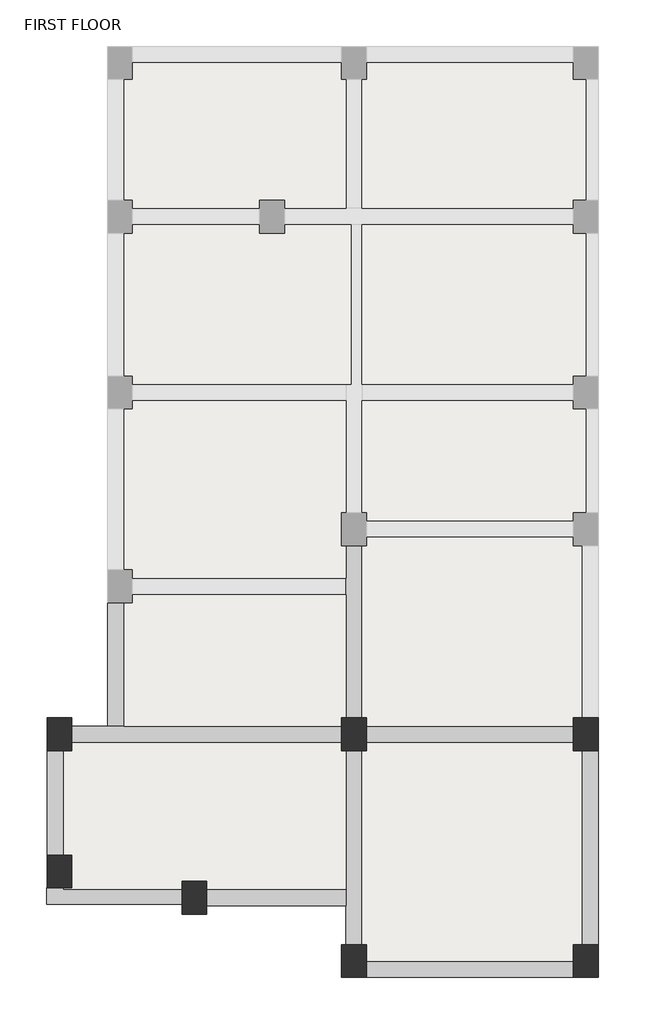
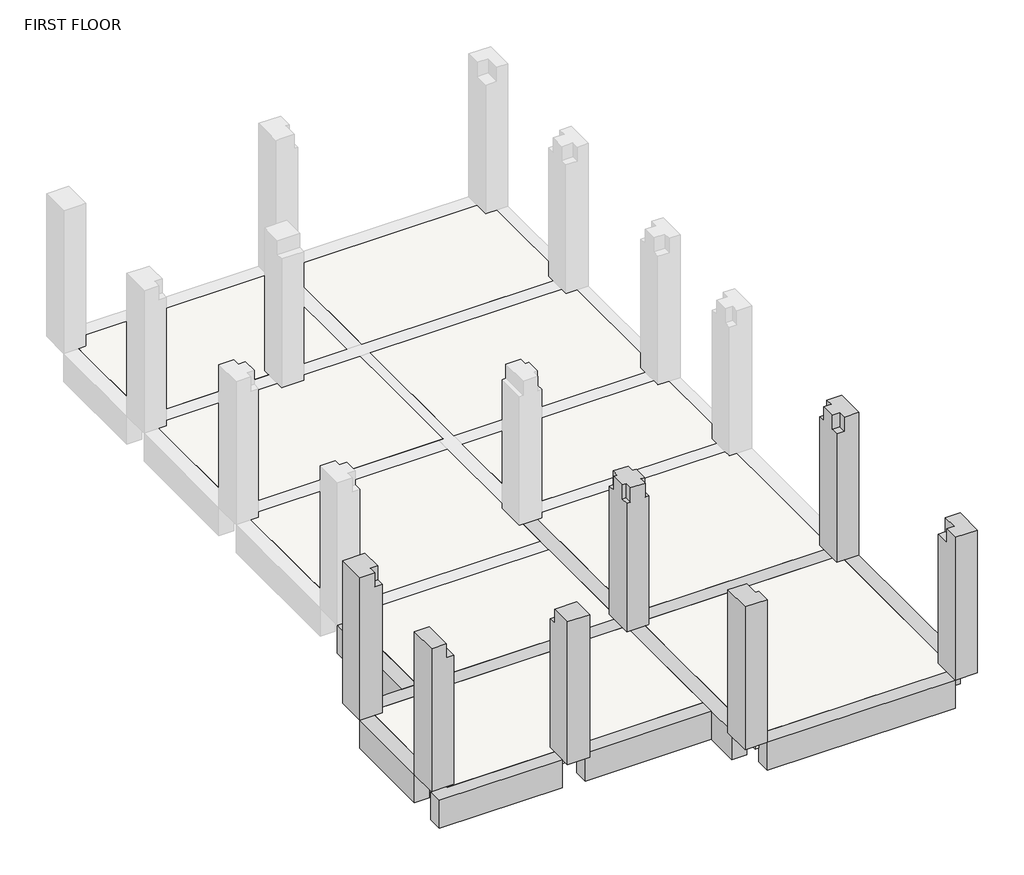
# One storey, part 1 of 2: 10 beams, 10 slabs, 7 columns.
"""IFC4 building model written with IfcOpenShell, lengths in millimetres."""

from ifc_helpers import new_model, si_unit, frame, origin, place, context, project, spatial, polyline, outline, extrude, faceted_brep, element, save

model = new_model("IFC4")

# Units and contexts
model_context = context("Model", 3, world=origin())
ifc_project = project(units=[si_unit("LENGTHUNIT", "METRE", prefix="MILLI")], contexts=[model_context])

# Site, building, storey
site = spatial("IfcSite", under=ifc_project)
building = spatial("IfcBuilding", under=site)
storey = spatial("IfcBuildingStorey", under=building, Name="FIRST FLOOR", Elevation=3000.0)

# Beams
placement = place(None, origin())
element("IfcBeam", 1, ObjectType="M_Concrete-Rectangular Beam : 300 x 600mm", at=placement, inside=storey, context=model_context, shape_type="SweptSolid", body=[
    extrude(outline(polyline([(2143.5134108, -6267.3380763), (2143.5134108, -6567.3380763), (-1646.635935, -6567.3380763), (-1646.635935, -6267.3380763), (2143.5134108, -6267.3380763)])), frame((0.0, 0.0, 2400.0), z_axis=(0.0, 0.0, 1.0), x_axis=(1.0, 0.0, 0.0)), (0.0, 0.0, 1.0), 600.0),
])
element("IfcBeam", 2, ObjectType="M_Concrete-Rectangular Beam : 300 x 600mm", at=placement, inside=storey, context=model_context, shape_type="SweptSolid", body=[
    extrude(outline(polyline([(2293.5134108, -2423.3693625), (2593.5134108, -2423.3693625), (2593.5134108, -5967.3380763), (2293.5134108, -5967.3380763), (2293.5134108, -2423.3693625)])), frame((0.0, 0.0, 2400.0), z_axis=(0.0, 0.0, 1.0), x_axis=(1.0, 0.0, 0.0)), (0.0, 0.0, 1.0), 600.0),
])
element("IfcBeam", 3, ObjectType="M_Concrete-Rectangular Beam : 300 x 600mm", at=placement, inside=storey, context=model_context, shape_type="SweptSolid", body=[
    extrude(outline(polyline([(-1646.635935, -2273.3693625), (-1646.635935, -1973.3693625), (2143.5134108, -1973.3693625), (2143.5134108, -2273.3693625), (-1646.635935, -2273.3693625)])), frame((0.0, 0.0, 2400.0), z_axis=(0.0, 0.0, 1.0), x_axis=(1.0, 0.0, 0.0)), (0.0, 0.0, 1.0), 600.0),
])
element("IfcBeam", 4, ObjectType="M_Concrete-Rectangular Beam : 300 x 600mm", at=placement, inside=storey, context=model_context, shape_type="Brep", body=[
    faceted_brep([(-1721.635935, -2423.3693625, 3000.0), (-2021.635935, -2423.3693625, 3000.0), (-2021.635935, -4959.2575036, 3000.0), (-2021.635935, -5259.2575036, 3000.0), (-2021.635935, -5967.3380763, 3000.0), (-1721.635935, -5967.3380763, 3000.0), (-1721.635935, -2423.3693625, 2400.0), (-1721.635935, -5967.3380763, 2400.0), (-2021.635935, -2423.3693625, 2400.0), (-2021.635935, -5967.3380763, 2400.0), (-2021.635935, -5259.2575036, 2400.0), (-2021.635935, -4959.2575036, 2400.0)], [[[0, 1, 2, 3, 4, 5]], [[6, 0, 5, 7]], [[8, 6, 7, 9, 10, 11]], [[1, 8, 11, 10, 9, 4, 3, 2]], [[1, 0, 6, 8]], [[4, 9, 7, 5]]]),
])
element("IfcBeam", 5, ObjectType="M_Concrete-Rectangular Beam : 300 x 600mm", at=placement, inside=storey, context=model_context, shape_type="Brep", body=[
    faceted_brep([(-1721.635935, 1328.1057379, 3000.0), (-2021.635935, 1328.1057379, 3000.0), (-2021.635935, 731.5941646, 3000.0), (-2021.635935, 431.5941646, 3000.0), (-2021.635935, -1823.3693625, 3000.0), (-1721.635935, -1823.3693625, 3000.0), (-1721.635935, 1328.1057379, 2400.0), (-1721.635935, -1823.3693625, 2400.0), (-2021.635935, 1328.1057379, 2400.0), (-2021.635935, -1823.3693625, 2400.0), (-2021.635935, 431.5941646, 2400.0), (-2021.635935, 731.5941646, 2400.0)], [[[0, 1, 2, 3, 4, 5]], [[6, 0, 5, 7]], [[8, 6, 7, 9, 10, 11]], [[1, 8, 11, 10, 9, 4, 3, 2]], [[1, 0, 6, 8]], [[4, 9, 7, 5]]]),
])
element("IfcBeam", 6, ObjectType="M_Concrete-Rectangular Beam : 300 x 600mm", at=placement, inside=storey, context=model_context, shape_type="Brep", body=[
    faceted_brep([(-4566.635935, -4959.2575036, 3000.0), (-4566.635935, -5259.2575036, 3000.0), (-2021.635935, -5259.2575036, 3000.0), (-2021.635935, -4959.2575036, 3000.0), (-4566.635935, -5259.2575036, 2400.0), (-2021.635935, -5259.2575036, 2400.0), (-4566.635935, -4959.2575036, 2400.0), (-2021.635935, -4959.2575036, 2400.0), (-2021.635935, -4959.2575036, 2700.0)], [[[0, 1, 2, 3]], [[1, 4, 5, 2]], [[4, 6, 7, 5]], [[6, 0, 3, 8, 7]], [[0, 6, 4, 1]], [[3, 2, 5, 7, 8]]]),
])
element("IfcBeam", 7, ObjectType="M_Concrete-Rectangular Beam : 300 x 600mm", at=placement, inside=storey, context=model_context, shape_type="Brep", body=[
    faceted_brep([(-7032.9642664, -1973.3693625, 3000.0), (-7032.9642664, -2273.3693625, 3000.0), (-2096.635935, -2273.3693625, 3000.0), (-2096.635935, -1973.3693625, 3000.0), (-6075.9642664, -1973.3693625, 3000.0), (-6375.9642664, -1973.3693625, 3000.0), (-7032.9642664, -1973.3693625, 2400.0), (-2096.635935, -1973.3693625, 2400.0), (-6075.9642664, -1973.3693625, 2400.0), (-6375.9642664, -1973.3693625, 2400.0), (-7032.9642664, -2273.3693625, 2400.0), (-2096.635935, -2273.3693625, 2400.0)], [[[0, 1, 2, 3, 4, 5]], [[6, 0, 5, 4, 3, 7, 8, 9]], [[10, 6, 9, 8, 7, 11]], [[1, 10, 11, 2]], [[2, 11, 7, 3]], [[1, 0, 6, 10]]]),
])
element("IfcBeam", 8, ObjectType="M_Concrete-Rectangular Beam : 300 x 600mm", at=placement, inside=storey, context=model_context, shape_type="Brep", body=[
    faceted_brep([(-6075.9642664, 281.5941646, 3000.0), (-6375.9642664, 281.5941646, 3000.0), (-6375.9642664, -1973.3693625, 3000.0), (-6075.9642664, -1973.3693625, 3000.0), (-6375.9642664, 281.5941646, 2400.0), (-6375.9642664, -1973.3693625, 2400.0), (-6075.9642664, 281.5941646, 2400.0), (-6075.9642664, -1973.3693625, 2400.0), (-6075.9642664, -1973.3693625, 2700.0)], [[[0, 1, 2, 3]], [[1, 4, 5, 2]], [[4, 6, 7, 5]], [[6, 0, 3, 8, 7]], [[0, 6, 4, 1]], [[3, 2, 5, 7, 8]]]),
])
element("IfcBeam", 9, ObjectType="M_Concrete-Rectangular Beam : 300 x 600mm", at=placement, inside=storey, context=model_context, shape_type="SweptSolid", body=[
    extrude(outline(polyline([(-7182.9642664, -4329.2575036), (-7482.9642664, -4329.2575036), (-7482.9642664, -2423.3693625), (-7182.9642664, -2423.3693625), (-7182.9642664, -4329.2575036)])), frame((0.0, 0.0, 2400.0), z_axis=(0.0, 0.0, 1.0), x_axis=(1.0, 0.0, 0.0)), (0.0, 0.0, 1.0), 600.0),
])
element("IfcBeam", 10, ObjectType="M_Concrete-Rectangular Beam : 300 x 600mm", at=placement, inside=storey, context=model_context, shape_type="Brep", body=[
    faceted_brep([(-7496.635935, -5229.2575036, 3000.0), (-7496.635935, -4929.2575036, 3000.0), (-7496.635935, -4929.2575036, 2400.0), (-7496.635935, -5229.2575036, 2400.0), (-5016.635935, -5229.2575036, 3000.0), (-5016.635935, -4959.2575036, 3000.0), (-7182.9642664, -4959.2575036, 3000.0), (-7182.9642664, -4929.2575036, 3000.0), (-7482.9642664, -4929.2575036, 3000.0), (-7182.9642664, -4929.2575036, 2700.0), (-7032.9642664, -4929.2575036, 2700.0), (-5016.635935, -4929.2575036, 2700.0), (-5016.635935, -4929.2575036, 2400.0), (-5016.635935, -5229.2575036, 2400.0), (-5016.635935, -4959.2575036, 2700.0), (-7182.9642664, -4959.2575036, 2700.0)], [[[0, 1, 2, 3]], [[1, 0, 4, 5, 6, 7, 8]], [[2, 1, 8, 7, 9, 10, 11, 12]], [[3, 2, 12, 13]], [[0, 3, 13, 4]], [[4, 13, 12, 11, 14, 5]], [[9, 15, 14, 11, 10]], [[15, 6, 5, 14]], [[6, 15, 9, 7]]]),
])

# Columns
element("IfcColumn", 11, ObjectType="M_Concrete-Rectangular-Column : 450 x 600mm", at=placement, inside=storey, context=model_context, shape_type="SweptSolid", body=[
    extrude(outline(polyline([(3000.0, -7482.9642664), (3000.0, -7032.9642664), (5748.0, -7032.9642664), (5748.0, -7182.9642664), (6048.0, -7182.9642664), (6048.0, -7482.9642664), (3000.0, -7482.9642664)])), frame((0.0, -4929.2575036, 0.0), z_axis=(0.0, 1.0, 0.0), x_axis=(0.0, 0.0, 1.0)), (0.0, 0.0, 1.0), 600.0),
])
element("IfcColumn", 12, ObjectType="M_Concrete-Rectangular-Column : 450 x 600mm", at=placement, inside=storey, context=model_context, shape_type="Brep", body=[
    faceted_brep([(-1646.635935, -1823.3693625, 3000.0), (-1646.635935, -2423.3693625, 3000.0), (-2096.635935, -2423.3693625, 3000.0), (-2096.635935, -1823.3693625, 3000.0), (-1646.635935, -1823.3693625, 5748.0), (-1646.635935, -1973.3693625, 5748.0), (-1646.635935, -1973.3693625, 6048.0), (-1646.635935, -2273.3693625, 6048.0), (-1646.635935, -2273.3693625, 5748.0), (-1646.635935, -2423.3693625, 5748.0), (-1721.635935, -2423.3693625, 5748.0), (-1721.635935, -2423.3693625, 6048.0), (-2021.635935, -2423.3693625, 6048.0), (-2021.635935, -2423.3693625, 5748.0), (-2096.635935, -2423.3693625, 5748.0), (-2096.635935, -2273.3693625, 5748.0), (-2096.635935, -2273.3693625, 6048.0), (-2096.635935, -1973.3693625, 6048.0), (-2096.635935, -1973.3693625, 5748.0), (-2096.635935, -1823.3693625, 5748.0), (-2021.635935, -1823.3693625, 5748.0), (-2021.635935, -1823.3693625, 6048.0), (-1721.635935, -1823.3693625, 6048.0), (-1721.635935, -1823.3693625, 5748.0), (-1721.635935, -1973.3693625, 6048.0), (-2021.635935, -1973.3693625, 6048.0), (-2021.635935, -2273.3693625, 6048.0), (-1721.635935, -2273.3693625, 6048.0), (-1721.635935, -1973.3693625, 5748.0), (-1721.635935, -2273.3693625, 5748.0), (-2021.635935, -1973.3693625, 5748.0), (-2021.635935, -2273.3693625, 5748.0)], [[[0, 1, 2, 3]], [[1, 0, 4, 5, 6, 7, 8, 9]], [[2, 1, 9, 10, 11, 12, 13, 14]], [[3, 2, 14, 15, 16, 17, 18, 19]], [[0, 3, 19, 20, 21, 22, 23, 4]], [[6, 24, 22, 21, 25, 17, 16, 26, 12, 11, 27, 7]], [[23, 28, 5, 4]], [[28, 24, 6, 5]], [[24, 28, 23, 22]], [[29, 10, 9, 8]], [[27, 29, 8, 7]], [[29, 27, 11, 10]], [[18, 30, 20, 19]], [[30, 25, 21, 20]], [[25, 30, 18, 17]], [[13, 31, 15, 14]], [[31, 26, 16, 15]], [[26, 31, 13, 12]]]),
])
element("IfcColumn", 13, ObjectType="M_Concrete-Rectangular-Column : 450 x 600mm", at=placement, inside=storey, context=model_context, shape_type="Brep", body=[
    faceted_brep([(-1646.635935, -5967.3380763, 3000.0), (-1646.635935, -6567.3380763, 3000.0), (-2096.635935, -6567.3380763, 3000.0), (-2096.635935, -5967.3380763, 3000.0), (-1646.635935, -5967.3380763, 5748.0), (-1646.635935, -6267.3380763, 5748.0), (-1646.635935, -6267.3380763, 6048.0), (-1646.635935, -6567.3380763, 6048.0), (-2096.635935, -6567.3380763, 6048.0), (-2096.635935, -5967.3380763, 6048.0), (-1721.635935, -5967.3380763, 6048.0), (-1721.635935, -5967.3380763, 5748.0), (-1721.635935, -6267.3380763, 6048.0), (-1721.635935, -6267.3380763, 5748.0)], [[[0, 1, 2, 3]], [[1, 0, 4, 5, 6, 7]], [[2, 1, 7, 8]], [[3, 2, 8, 9]], [[0, 3, 9, 10, 11, 4]], [[8, 7, 6, 12, 10, 9]], [[11, 13, 5, 4]], [[13, 12, 6, 5]], [[12, 13, 11, 10]]]),
])
element("IfcColumn", 14, ObjectType="M_Concrete-Rectangular-Column : 450 x 600mm", at=placement, inside=storey, context=model_context, shape_type="Brep", body=[
    faceted_brep([(2593.5134108, -1823.3693625, 3000.0), (2593.5134108, -2423.3693625, 3000.0), (2143.5134108, -2423.3693625, 3000.0), (2143.5134108, -1823.3693625, 3000.0), (2593.5134108, -1823.3693625, 6048.0), (2593.5134108, -2423.3693625, 6048.0), (2293.5134108, -2423.3693625, 6048.0), (2293.5134108, -2423.3693625, 5748.0), (2143.5134108, -2423.3693625, 5748.0), (2143.5134108, -2273.3693625, 5748.0), (2143.5134108, -2273.3693625, 6048.0), (2143.5134108, -1973.3693625, 6048.0), (2143.5134108, -1973.3693625, 5748.0), (2143.5134108, -1823.3693625, 5748.0), (2293.5134108, -1823.3693625, 5748.0), (2293.5134108, -1823.3693625, 6048.0), (2293.5134108, -1973.3693625, 6048.0), (2293.5134108, -2273.3693625, 6048.0), (2293.5134108, -1973.3693625, 5748.0), (2293.5134108, -2273.3693625, 5748.0)], [[[0, 1, 2, 3]], [[1, 0, 4, 5]], [[2, 1, 5, 6, 7, 8]], [[3, 2, 8, 9, 10, 11, 12, 13]], [[0, 3, 13, 14, 15, 4]], [[5, 4, 15, 16, 11, 10, 17, 6]], [[12, 18, 14, 13]], [[18, 16, 15, 14]], [[16, 18, 12, 11]], [[7, 19, 9, 8]], [[19, 17, 10, 9]], [[17, 19, 7, 6]]]),
])
element("IfcColumn", 15, ObjectType="M_Concrete-Rectangular-Column : 450 x 600mm", at=placement, inside=storey, context=model_context, shape_type="Brep", body=[
    faceted_brep([(2593.5134108, -5967.3380763, 3000.0), (2593.5134108, -6567.3380763, 3000.0), (2143.5134108, -6567.3380763, 3000.0), (2143.5134108, -5967.3380763, 3000.0), (2593.5134108, -5967.3380763, 6048.0), (2593.5134108, -6567.3380763, 6048.0), (2143.5134108, -6567.3380763, 6048.0), (2143.5134108, -6267.3380763, 6048.0), (2143.5134108, -6267.3380763, 5748.0), (2143.5134108, -5967.3380763, 5748.0), (2293.5134108, -5967.3380763, 5748.0), (2293.5134108, -5967.3380763, 6048.0), (2293.5134108, -6267.3380763, 6048.0), (2293.5134108, -6267.3380763, 5748.0)], [[[0, 1, 2, 3]], [[1, 0, 4, 5]], [[2, 1, 5, 6]], [[3, 2, 6, 7, 8, 9]], [[0, 3, 9, 10, 11, 4]], [[5, 4, 11, 12, 7, 6]], [[8, 13, 10, 9]], [[13, 12, 11, 10]], [[12, 13, 8, 7]]]),
])
element("IfcColumn", 16, ObjectType="M_Concrete-Rectangular-Column : 450 x 600mm", at=placement, inside=storey, context=model_context, shape_type="SweptSolid", body=[
    extrude(outline(polyline([(-4809.2575036, 3000.0), (-5409.2575036, 3000.0), (-5409.2575036, 6048.0), (-4959.2575036, 6048.0), (-4959.2575036, 5748.0), (-4809.2575036, 5748.0), (-4809.2575036, 3000.0)])), frame((-5016.635935, 0.0, 0.0), z_axis=(1.0, 0.0, 0.0), x_axis=(0.0, 1.0, 0.0)), (0.0, 0.0, 1.0), 450.0),
])
element("IfcColumn", 17, ObjectType="M_Concrete-Rectangular-Column : 450 x 600mm", at=placement, inside=storey, context=model_context, shape_type="Brep", body=[
    faceted_brep([(-7032.9642664, -1823.3693625, 3000.0), (-7032.9642664, -2423.3693625, 3000.0), (-7482.9642664, -2423.3693625, 3000.0), (-7482.9642664, -1823.3693625, 3000.0), (-7032.9642664, -1823.3693625, 6048.0), (-7032.9642664, -2273.3693625, 6048.0), (-7032.9642664, -2273.3693625, 5748.0), (-7032.9642664, -2423.3693625, 5748.0), (-7182.9642664, -2423.3693625, 5748.0), (-7182.9642664, -2423.3693625, 6048.0), (-7482.9642664, -2423.3693625, 6048.0), (-7482.9642664, -1823.3693625, 6048.0), (-7182.9642664, -2273.3693625, 6048.0), (-7182.9642664, -2273.3693625, 5748.0)], [[[0, 1, 2, 3]], [[1, 0, 4, 5, 6, 7]], [[2, 1, 7, 8, 9, 10]], [[3, 2, 10, 11]], [[0, 3, 11, 4]], [[11, 10, 9, 12, 5, 4]], [[13, 8, 7, 6]], [[12, 13, 6, 5]], [[13, 12, 9, 8]]]),
])

# Slabs
element("IfcSlab", 18, ObjectType="Generic 300mm", at=placement, inside=storey, context=model_context, shape_type="SweptSolid", body=[
    extrude(outline(polyline([(-2096.635935, 10150.0657956), (-2096.635935, 9850.0657956), (-2021.635935, 9850.0657956), (-2021.635935, 7491.506653), (-3146.635935, 7491.506653), (-3146.635935, 7641.506653), (-3596.635935, 7641.506653), (-3596.635935, 7491.506653), (-5925.9642664, 7491.506653), (-5925.9642664, 7641.506653), (-6075.9642664, 7641.506653), (-6075.9642664, 9850.0657956), (-5925.9642664, 9850.0657956), (-5925.9642664, 10150.0657956), (-2096.635935, 10150.0657956)])), frame((0.0, 0.0, 2700.0), z_axis=(0.0, 0.0, 1.0), x_axis=(1.0, 0.0, 0.0)), (0.0, 0.0, 1.0), 300.0),
])
element("IfcSlab", 19, ObjectType="Generic 300mm", at=placement, inside=storey, context=model_context, shape_type="Brep", body=[
    faceted_brep([(-1721.635935, 10150.0657956, 2700.0), (-1646.635935, 10150.0657956, 2700.0), (2143.5134108, 10150.0657956, 2700.0), (2368.5134108, 10150.0657956, 2700.0), (2368.5134108, 9850.0657956, 2700.0), (2368.5134108, 7641.506653, 2700.0), (2368.5134108, 7491.506653, 2700.0), (2143.5134108, 7491.506653, 2700.0), (-1721.635935, 7491.506653, 2700.0), (-1721.635935, 9850.0657956, 2700.0), (-1721.635935, 10150.0657956, 3000.0), (-1721.635935, 9850.0657956, 3000.0), (-1721.635935, 7491.506653, 3000.0), (2143.5134108, 7491.506653, 3000.0), (2368.5134108, 7491.506653, 3000.0), (2368.5134108, 7641.506653, 3000.0), (2368.5134108, 9850.0657956, 3000.0), (2368.5134108, 10150.0657956, 3000.0), (2143.5134108, 10150.0657956, 3000.0), (-1646.635935, 10150.0657956, 3000.0)], [[[0, 1, 2, 3, 4, 5, 6, 7, 8, 9]], [[10, 11, 12, 13, 14, 15, 16, 17, 18, 19]], [[3, 2, 1, 0, 10, 19, 18, 17]], [[6, 5, 4, 3, 17, 16, 15, 14]], [[8, 7, 6, 14, 13, 12]], [[0, 9, 8, 12, 11, 10]]]),
])
element("IfcSlab", 20, ObjectType="Generic 300mm", at=placement, inside=storey, context=model_context, shape_type="Brep", body=[
    faceted_brep([(-1721.635935, 7191.506653, 2700.0), (2143.5134108, 7191.506653, 2700.0), (2368.5134108, 7191.506653, 2700.0), (2368.5134108, 7041.506653, 2700.0), (2368.5134108, 4424.5351605, 2700.0), (2368.5134108, 4274.5351605, 2700.0), (2143.5134108, 4274.5351605, 2700.0), (-1721.635935, 4274.5351605, 2700.0), (-1721.635935, 7191.506653, 3000.0), (-1721.635935, 4274.5351605, 3000.0), (2143.5134108, 4274.5351605, 3000.0), (2368.5134108, 4274.5351605, 3000.0), (2368.5134108, 4424.5351605, 3000.0), (2368.5134108, 7041.506653, 3000.0), (2368.5134108, 7191.506653, 3000.0), (2143.5134108, 7191.506653, 3000.0)], [[[0, 1, 2, 3, 4, 5, 6, 7]], [[8, 9, 10, 11, 12, 13, 14, 15]], [[2, 1, 0, 8, 15, 14]], [[5, 4, 3, 2, 14, 13, 12, 11]], [[7, 6, 5, 11, 10, 9]], [[0, 7, 9, 8]]]),
])
element("IfcSlab", 21, ObjectType="Generic 300mm", at=placement, inside=storey, context=model_context, shape_type="Brep", body=[
    faceted_brep([(-6075.9642664, 7191.506653, 2700.0), (-5925.9642664, 7191.506653, 2700.0), (-3596.635935, 7191.506653, 2700.0), (-3146.635935, 7191.506653, 2700.0), (-2021.635935, 7191.506653, 2700.0), (-1928.7254278, 7191.506653, 2700.0), (-1928.7254278, 4274.5351605, 2700.0), (-2021.635935, 4274.5351605, 2700.0), (-5925.9642664, 4274.5351605, 2700.0), (-6075.9642664, 4274.5351605, 2700.0), (-6075.9642664, 4424.5351605, 2700.0), (-6075.9642664, 7041.506653, 2700.0), (-6075.9642664, 7191.506653, 3000.0), (-6075.9642664, 7041.506653, 3000.0), (-6075.9642664, 4424.5351605, 3000.0), (-6075.9642664, 4274.5351605, 3000.0), (-5925.9642664, 4274.5351605, 3000.0), (-2021.635935, 4274.5351605, 3000.0), (-1928.7254278, 4274.5351605, 3000.0), (-1928.7254278, 7191.506653, 3000.0), (-3146.635935, 7191.506653, 3000.0), (-3596.635935, 7191.506653, 3000.0), (-5925.9642664, 7191.506653, 3000.0)], [[[0, 1, 2, 3, 4, 5, 6, 7, 8, 9, 10, 11]], [[12, 13, 14, 15, 16, 17, 18, 19, 20, 21, 22]], [[5, 4, 3, 2, 1, 0, 12, 22, 21, 20, 19]], [[6, 5, 19, 18]], [[9, 8, 7, 6, 18, 17, 16, 15]], [[0, 11, 10, 9, 15, 14, 13, 12]]]),
])
element("IfcSlab", 22, ObjectType="Generic 300mm", at=placement, inside=storey, context=model_context, shape_type="Brep", body=[
    faceted_brep([(-1721.635935, 3974.5351605, 2700.0), (2143.5134108, 3974.5351605, 2700.0), (2368.5134108, 3974.5351605, 2700.0), (2368.5134108, 3824.5351605, 2700.0), (2368.5134108, 1928.1057379, 2700.0), (2368.5134108, 1778.1057379, 2700.0), (2143.5134108, 1778.1057379, 2700.0), (-1646.635935, 1778.1057379, 2700.0), (-1721.635935, 1778.1057379, 2700.0), (-1721.635935, 1928.1057379, 2700.0), (-1721.635935, 3974.5351605, 3000.0), (-1721.635935, 1928.1057379, 3000.0), (-1721.635935, 1778.1057379, 3000.0), (-1646.635935, 1778.1057379, 3000.0), (2143.5134108, 1778.1057379, 3000.0), (2368.5134108, 1778.1057379, 3000.0), (2368.5134108, 1928.1057379, 3000.0), (2368.5134108, 3824.5351605, 3000.0), (2368.5134108, 3974.5351605, 3000.0), (2143.5134108, 3974.5351605, 3000.0)], [[[0, 1, 2, 3, 4, 5, 6, 7, 8, 9]], [[10, 11, 12, 13, 14, 15, 16, 17, 18, 19]], [[2, 1, 0, 10, 19, 18]], [[5, 4, 3, 2, 18, 17, 16, 15]], [[8, 7, 6, 5, 15, 14, 13, 12]], [[0, 9, 8, 12, 11, 10]]]),
])
element("IfcSlab", 23, ObjectType="Generic 300mm", at=placement, inside=storey, context=model_context, shape_type="Brep", body=[
    faceted_brep([(-1721.635935, 1478.1057379, 2700.0), (-1646.635935, 1478.1057379, 2700.0), (2143.5134108, 1478.1057379, 2700.0), (2293.5134108, 1478.1057379, 2700.0), (2293.5134108, 1328.1057379, 2700.0), (2293.5134108, -1823.3693625, 2700.0), (2293.5134108, -1973.3693625, 2700.0), (2143.5134108, -1973.3693625, 2700.0), (-1646.635935, -1973.3693625, 2700.0), (-1721.635935, -1973.3693625, 2700.0), (-1721.635935, -1823.3693625, 2700.0), (-1721.635935, 1328.1057379, 2700.0), (-1721.635935, 1478.1057379, 3000.0), (-1721.635935, 1328.1057379, 3000.0), (-1721.635935, -1823.3693625, 3000.0), (-1721.635935, -1973.3693625, 3000.0), (-1646.635935, -1973.3693625, 3000.0), (2143.5134108, -1973.3693625, 3000.0), (2293.5134108, -1973.3693625, 3000.0), (2293.5134108, -1823.3693625, 3000.0), (2293.5134108, 1328.1057379, 3000.0), (2293.5134108, 1478.1057379, 3000.0), (2143.5134108, 1478.1057379, 3000.0), (-1646.635935, 1478.1057379, 3000.0)], [[[0, 1, 2, 3, 4, 5, 6, 7, 8, 9, 10, 11]], [[12, 13, 14, 15, 16, 17, 18, 19, 20, 21, 22, 23]], [[3, 2, 1, 0, 12, 23, 22, 21]], [[6, 5, 4, 3, 21, 20, 19, 18]], [[9, 8, 7, 6, 18, 17, 16, 15]], [[0, 11, 10, 9, 15, 14, 13, 12]]]),
])
element("IfcSlab", 24, ObjectType="Generic 300mm", at=placement, inside=storey, context=model_context, shape_type="Brep", body=[
    faceted_brep([(-1721.635935, -2273.3693625, 2700.0), (-1646.635935, -2273.3693625, 2700.0), (2143.5134108, -2273.3693625, 2700.0), (2293.5134108, -2273.3693625, 2700.0), (2293.5134108, -2423.3693625, 2700.0), (2293.5134108, -5967.3380763, 2700.0), (2293.5134108, -6267.3380763, 2700.0), (2143.5134108, -6267.3380763, 2700.0), (-1646.635935, -6267.3380763, 2700.0), (-1721.635935, -6267.3380763, 2700.0), (-1721.635935, -5967.3380763, 2700.0), (-1721.635935, -2423.3693625, 2700.0), (-1721.635935, -2273.3693625, 3000.0), (-1721.635935, -2423.3693625, 3000.0), (-1721.635935, -5967.3380763, 3000.0), (-1721.635935, -6267.3380763, 3000.0), (-1646.635935, -6267.3380763, 3000.0), (2143.5134108, -6267.3380763, 3000.0), (2293.5134108, -6267.3380763, 3000.0), (2293.5134108, -5967.3380763, 3000.0), (2293.5134108, -2423.3693625, 3000.0), (2293.5134108, -2273.3693625, 3000.0), (2143.5134108, -2273.3693625, 3000.0), (-1646.635935, -2273.3693625, 3000.0)], [[[0, 1, 2, 3, 4, 5, 6, 7, 8, 9, 10, 11]], [[12, 13, 14, 15, 16, 17, 18, 19, 20, 21, 22, 23]], [[3, 2, 1, 0, 12, 23, 22, 21]], [[6, 5, 4, 3, 21, 20, 19, 18]], [[9, 8, 7, 6, 18, 17, 16, 15]], [[0, 11, 10, 9, 15, 14, 13, 12]]]),
])
element("IfcSlab", 25, ObjectType="Generic 300mm", at=placement, inside=storey, context=model_context, shape_type="Brep", body=[
    faceted_brep([(-6075.9642664, 3974.5351605, 2700.0), (-5925.9642664, 3974.5351605, 2700.0), (-2021.635935, 3974.5351605, 2700.0), (-2021.635935, 1928.1057379, 2700.0), (-2021.635935, 1328.1057379, 2700.0), (-2021.635935, 731.5941646, 2700.0), (-5925.9642664, 731.5941646, 2700.0), (-6075.9642664, 731.5941646, 2700.0), (-6075.9642664, 881.5941646, 2700.0), (-6075.9642664, 3824.5351605, 2700.0), (-6075.9642664, 3974.5351605, 3000.0), (-6075.9642664, 3824.5351605, 3000.0), (-6075.9642664, 881.5941646, 3000.0), (-6075.9642664, 731.5941646, 3000.0), (-5925.9642664, 731.5941646, 3000.0), (-2021.635935, 731.5941646, 3000.0), (-2021.635935, 1328.1057379, 3000.0), (-2021.635935, 1928.1057379, 3000.0), (-2021.635935, 3974.5351605, 3000.0), (-5925.9642664, 3974.5351605, 3000.0)], [[[0, 1, 2, 3, 4, 5, 6, 7, 8, 9]], [[10, 11, 12, 13, 14, 15, 16, 17, 18, 19]], [[2, 1, 0, 10, 19, 18]], [[5, 4, 3, 2, 18, 17, 16, 15]], [[7, 6, 5, 15, 14, 13]], [[0, 9, 8, 7, 13, 12, 11, 10]]]),
])
element("IfcSlab", 26, ObjectType="Generic 300mm", at=placement, inside=storey, context=model_context, shape_type="Brep", body=[
    faceted_brep([(-6075.9642664, 431.5941646, 2700.0), (-5925.9642664, 431.5941646, 2700.0), (-2021.635935, 431.5941646, 2700.0), (-2021.635935, -1823.3693625, 2700.0), (-2021.635935, -1973.3693625, 2700.0), (-2096.635935, -1973.3693625, 2700.0), (-6075.9642664, -1973.3693625, 2700.0), (-6075.9642664, 281.5941646, 2700.0), (-6075.9642664, 431.5941646, 3000.0), (-6075.9642664, 281.5941646, 3000.0), (-6075.9642664, -1973.3693625, 3000.0), (-2096.635935, -1973.3693625, 3000.0), (-2021.635935, -1973.3693625, 3000.0), (-2021.635935, -1823.3693625, 3000.0), (-2021.635935, 431.5941646, 3000.0), (-5925.9642664, 431.5941646, 3000.0)], [[[0, 1, 2, 3, 4, 5, 6, 7]], [[8, 9, 10, 11, 12, 13, 14, 15]], [[2, 1, 0, 8, 15, 14]], [[4, 3, 2, 14, 13, 12]], [[6, 5, 4, 12, 11, 10]], [[0, 7, 6, 10, 9, 8]]]),
])
element("IfcSlab", 27, ObjectType="Generic 300mm", at=placement, inside=storey, context=model_context, shape_type="Brep", body=[
    faceted_brep([(-7182.9642664, -2273.3693625, 2700.0), (-7032.9642664, -2273.3693625, 2700.0), (-2096.635935, -2273.3693625, 2700.0), (-2021.635935, -2273.3693625, 2700.0), (-2021.635935, -2423.3693625, 2700.0), (-2021.635935, -4959.2575036, 2700.0), (-4566.635935, -4959.2575036, 2700.0), (-5016.635935, -4959.2575036, 2700.0), (-7182.9642664, -4959.2575036, 2700.0), (-7182.9642664, -4929.2575036, 2700.0), (-7182.9642664, -4329.2575036, 2700.0), (-7182.9642664, -2423.3693625, 2700.0), (-7182.9642664, -2273.3693625, 3000.0), (-7182.9642664, -2423.3693625, 3000.0), (-7182.9642664, -4329.2575036, 3000.0), (-7182.9642664, -4929.2575036, 3000.0), (-7182.9642664, -4959.2575036, 3000.0), (-5016.635935, -4959.2575036, 3000.0), (-4566.635935, -4959.2575036, 3000.0), (-2021.635935, -4959.2575036, 3000.0), (-2021.635935, -2423.3693625, 3000.0), (-2021.635935, -2273.3693625, 3000.0), (-2096.635935, -2273.3693625, 3000.0), (-7032.9642664, -2273.3693625, 3000.0)], [[[0, 1, 2, 3, 4, 5, 6, 7, 8, 9, 10, 11]], [[12, 13, 14, 15, 16, 17, 18, 19, 20, 21, 22, 23]], [[3, 2, 1, 0, 12, 23, 22, 21]], [[5, 4, 3, 21, 20, 19]], [[8, 7, 6, 5, 19, 18, 17, 16]], [[0, 11, 10, 9, 8, 16, 15, 14, 13, 12]]]),
])

save(model, "model.ifc")

# Revit data of these elements
# Type "M_Concrete-Rectangular Beam : 300 x 600mm"
#   Length [instance default] = 1524 mm
#   b = 300 mm
#   h = 600 mm
#   Structural Material [instance default] = Concrete, Cast-in-Place gray
#   Assembly Code = ""
# Type "M_Concrete-Rectangular-Column : 450 x 600mm"
#   b = 450 mm
#   h = 600 mm
#   Structural Material [instance default] = Concrete, Cast-in-Place gray
# Type "Generic 300mm"
#   Function = 0
#   Layers, outside or top first: 300 mm no material (function 1)
# Elements 1, 2, 3, 4, 5, 6, 7, 8, 9, 10 (IfcBeam, "M_Concrete-Rectangular Beam : 300 x 600mm")
#   Structural Material = Concrete, Cast-in-Place gray
#   Phase Created = New Construction
#   Materials on its faces: "Concrete, Cast-in-Place gray"
# Elements 11, 12, 13, 14, 15, 16, 17 (IfcColumn, "M_Concrete-Rectangular-Column : 450 x 600mm")
#   Structural Material = Concrete, Cast-in-Place gray
#   Phase Created = New Construction
#   Materials on its faces: "Concrete, Cast-in-Place gray"
# Element 18 (IfcSlab, "Generic 300mm")
#   Height Offset From Level = 0 mm
#   built-in parameter 1001954 = 1
#   Phase Created = New Construction
#   Materials on its faces: "Default Floor"
# Elements 19, 20, 21, 22, 23, 24, 25, 26, 27 (IfcSlab, "Generic 300mm")
#   built-in parameter 1001955 = 3.14159 (stored number, unit not read)
#   Height Offset From Level = 0 mm
#   built-in parameter 1001954 = 1
#   Phase Created = New Construction
#   Materials on its faces: "Default Floor"
# Materials
#   "Concrete, Cast-in-Place gray": class "Concrete", colour RGB 192 192 192, transparency 0, Description = "Cast-in-place concrete", Cost = 0
#   "Default Floor": colour RGB 127 127 127, transparency 0, Cost = 0
